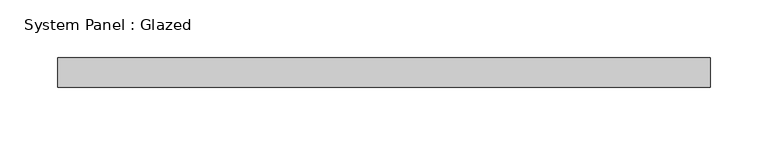
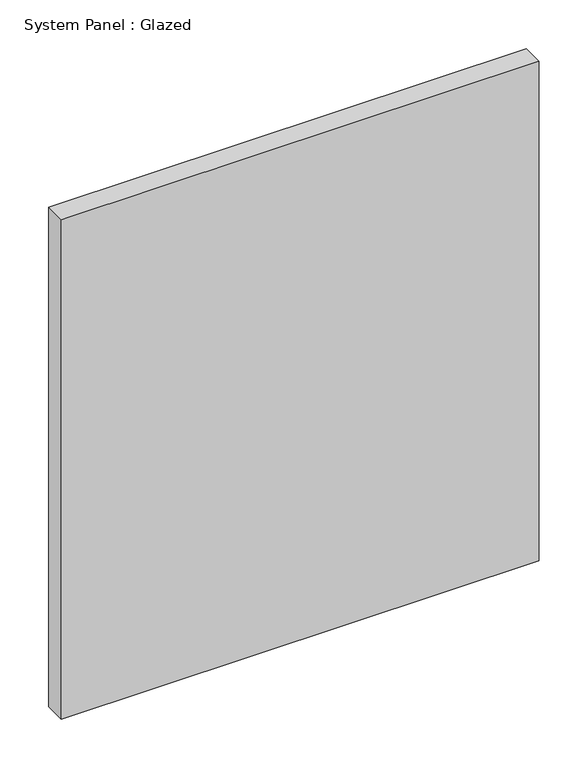
"""IFC4 building model written with IfcOpenShell, lengths in millimetres: plate geometry, System Panel : Glazed."""

from ifc_helpers import new_model, si_unit, origin, origin_with_axes, place, context, project, spatial, polyline, outline, extrude, source, transform, mapped, element, save


def system_panel_glazed_5721f284(model_context):
    return source(origin(), model_context, "Body", "SweptSolid", [
        extrude(outline(polyline([(282.575, 19.05), (-282.575, 19.05), (-282.575, 44.45), (282.575, 44.45), (282.575, 19.05)])), origin_with_axes(), (0.0, 0.0, 1.0), 624.3539078),
    ])


if __name__ == "__main__":
    model = new_model("IFC4")
    model_context = context("Model", 3, world=origin())
    ifc_project = project(units=[si_unit("LENGTHUNIT", "METRE", prefix="MILLI")], contexts=[model_context])
    site = spatial("IfcSite", under=ifc_project)
    building = spatial("IfcBuilding", under=site)
    placement = place(None, origin())
    system_panel_glazed_shape = system_panel_glazed_5721f284(model_context)
    element("IfcPlate", 1, ObjectType="System Panel : Glazed", at=placement, inside=building, context=model_context, shape_type="MappedRepresentation", body=[
        mapped(system_panel_glazed_shape, transform((0.0, 0.0, 0.0), x_axis=(1.0, 0.0, 0.0), y_axis=(0.0, 1.0, 0.0), z_axis=(0.0, 0.0, 1.0))),
    ])
    save(model, "model.ifc")

# Revit data of these elements
# Type "System Panel : Glazed"
#   Construction Type Id = "GSP4R"
#   Analytic Construction = "1/8 in Pilkington single glazing"
#   Visual Light Transmittance = 0.9
#   Solar Heat Gain Coefficient = 0.86
#   Heat Transfer Coefficient (U) = 1.18115 BTU/(h·ft²·°F)
#   Define Thermal Properties by = 1
# Element 1 (IfcPlate, "System Panel : Glazed")
#   Materials on its faces: "Glass"
# Materials
#   "Glass": class "Glass", colour RGB 0 128 192, transparency 0.75, Description = "Soda Lime Glass", Cost = 0
